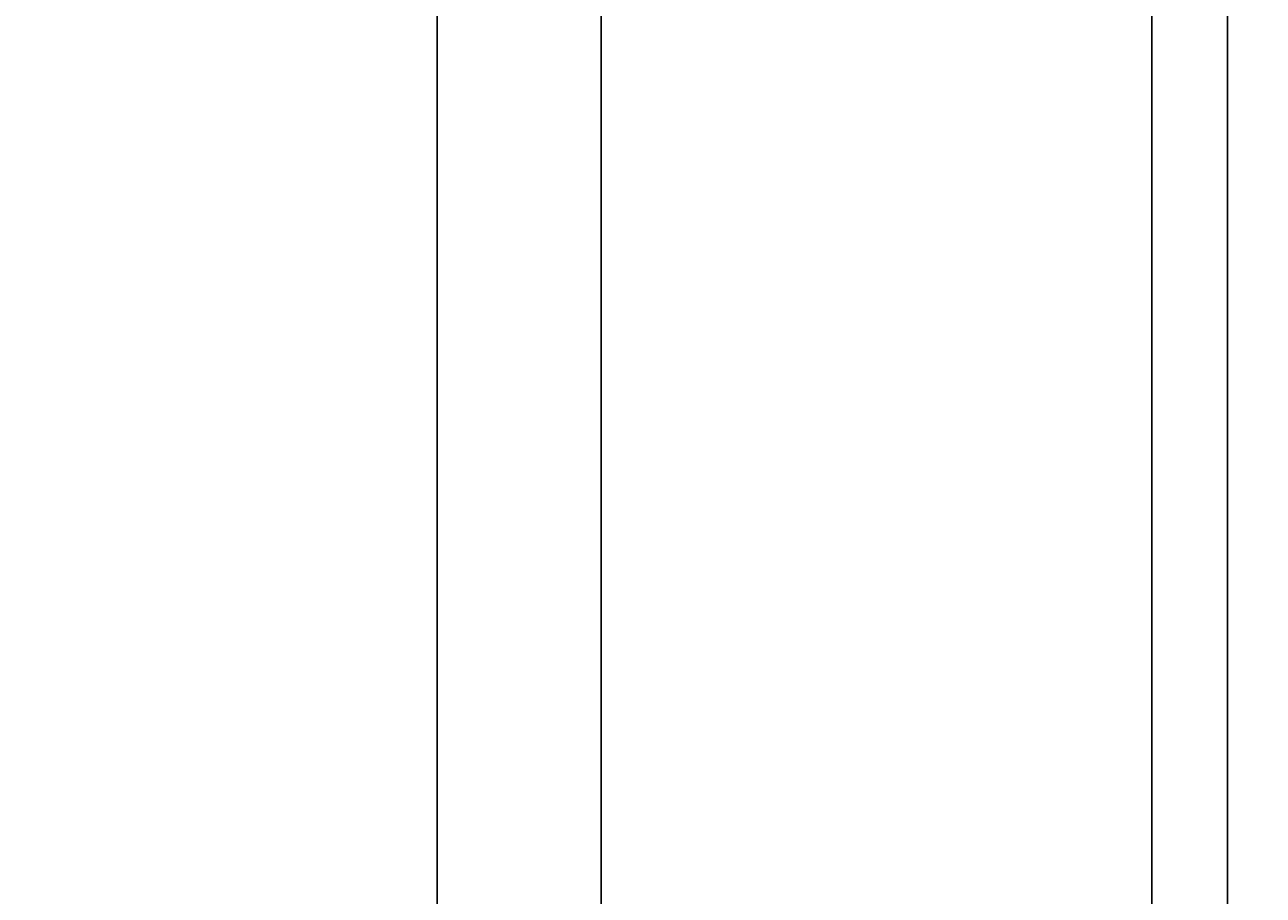
# Model space of a CAD drawing. Units: inches. Extents: x 35362 to 73946, y 43607 to 67532.
# Tile 123 of 134: x 50761 to 51337, y 49329 to 49735. Entities that reach past the tile are written whole.
import ezdxf

# ---------------------------------------------------------------- set-up
doc = ezdxf.new("R2010")
doc.units = ezdxf.units.IN
doc.header["$MEASUREMENT"] = 0
doc.layers.add('A-ANNO-DIMS', color=2, linetype='Continuous', lineweight=18)
doc.styles.get("Standard").update_dxf_attribs({"font": 'arial.ttf'})
doc.dimstyles.get("Standard").update_dxf_attribs({"dimtxt": 0.18, "dimasz": 0.18, "dimexe": 0.18, "dimexo": 0.0625, "dimgap": 0.09, "dimtad": 0, "dimtih": 1, "dimtoh": 1, "dimdec": 4, "dimzin": 0, "dimdsep": 46, "dimtxsty": 'Standard', "dimcen": 0.09, "dimadec": 0, "dimazin": 0, "dimtfac": 1, "dimtdec": 4, "dimtofl": 0, "dimtmove": 0, "dimatfit": 3, "dimfxl": 1, "dimtolj": 1, "dimtzin": 0, "dimarcsym": 0})

# ---------------------------------------------------------------- blocks, each defined once
blk = doc.blocks.new('*D11')
at = {"layer": 'A-ANNO-DIMS', "color": 0, "lineweight": -2, "transparency": 16777216}
for p, q in [((47978.66, 56028.77), (47978.66, 43606.68)), ((53109.76, 56028.77), (53109.76, 43606.68)), ((47978.84, 43606.86), (50543.87, 43606.86)), ((53109.58, 43606.86), (50544.55, 43606.86))]:
    blk.add_line(p, q, dxfattribs=at)
at = {"layer": 'A-ANNO-DIMS', "color": 0, "transparency": 16777216}
for points in [[(47978.84, 43606.89), (47978.84, 43606.83), (47978.66, 43606.86)], [(53109.58, 43606.89), (53109.58, 43606.83), (53109.76, 43606.86)]]:
    blk.add_solid(points, dxfattribs=at)
at = {"layer": 'Defpoints', "color": 0, "transparency": 16777216}
for p in [(47978.66, 56028.84), (53109.76, 56028.84), (53109.76, 43606.86)]:
    blk.add_point(p, dxfattribs=at)
at = {"layer": 'A-ANNO-DIMS', "color": 0, "transparency": 16777216, "insert": (50544.21, 43606.86), "char_height": 0.18, "attachment_point": 5}
blk.add_mtext('\\A1;5131', dxfattribs=at)
blk = doc.blocks.new('*D13')
at = {"layer": 'A-ANNO-DIMS', "color": 0, "lineweight": -2, "transparency": 16777216}
for p, q in [((48373.49, 51694.02), (48373.49, 43606.68)), ((51029.04, 51694.02), (51029.04, 43606.68)), ((48373.67, 43606.86), (49700.8, 43606.86)), ((51028.86, 43606.86), (49701.73, 43606.86))]:
    blk.add_line(p, q, dxfattribs=at)
at = {"layer": 'A-ANNO-DIMS', "color": 0, "transparency": 16777216}
for points in [[(48373.67, 43606.89), (48373.67, 43606.83), (48373.49, 43606.86)], [(51028.86, 43606.89), (51028.86, 43606.83), (51029.04, 43606.86)]]:
    blk.add_solid(points, dxfattribs=at)
at = {"layer": 'Defpoints', "color": 0, "transparency": 16777216}
for p in [(48373.49, 51694.09), (51029.04, 51694.09), (51029.04, 43606.86)]:
    blk.add_point(p, dxfattribs=at)
at = {"layer": 'A-ANNO-DIMS', "color": 0, "transparency": 16777216, "insert": (49701.27, 43606.86), "char_height": 0.18, "attachment_point": 5}
blk.add_mtext('\\A1;2655.6', dxfattribs=at)
blk = doc.blocks.new('*D17')
at = {"layer": 'A-ANNO-DIMS', "color": 0, "lineweight": -2, "transparency": 16777216}
for p, q in [((49923.31, 61293.22), (49923.31, 43606.68)), ((51913.93, 61293.22), (51913.93, 43606.68)), ((49923.49, 43606.86), (50918.16, 43606.86)), ((51913.75, 43606.86), (50919.07, 43606.86))]:
    blk.add_line(p, q, dxfattribs=at)
at = {"layer": 'A-ANNO-DIMS', "color": 0, "transparency": 16777216}
for points in [[(49923.49, 43606.89), (49923.49, 43606.83), (49923.31, 43606.86)], [(51913.75, 43606.89), (51913.75, 43606.83), (51913.93, 43606.86)]]:
    blk.add_solid(points, dxfattribs=at)
at = {"layer": 'Defpoints', "color": 0, "transparency": 16777216}
for p in [(49923.31, 61293.29), (51913.93, 61293.29), (51913.93, 43606.86)]:
    blk.add_point(p, dxfattribs=at)
at = {"layer": 'A-ANNO-DIMS', "color": 0, "transparency": 16777216, "insert": (50918.62, 43606.86), "char_height": 0.18, "attachment_point": 5}
blk.add_mtext('\\A1;1990.6', dxfattribs=at)
blk = doc.blocks.new('*D40')
at = {"layer": 'A-ANNO-DIMS', "color": 0, "lineweight": -2, "transparency": 16777216}
for p, q in [((56873.54, 53351.53), (35361.77, 53351.53)), ((35361.95, 53351.35), (35361.95, 51333.28)), ((35361.95, 49314.85), (35361.95, 51332.92)), ((51806.45, 49314.67), (35361.77, 49314.67))]:
    blk.add_line(p, q, dxfattribs=at)
at = {"layer": 'A-ANNO-DIMS', "color": 0, "transparency": 16777216}
for points in [[(35361.92, 53351.35), (35361.98, 53351.35), (35361.95, 53351.53)], [(35361.92, 49314.85), (35361.98, 49314.85), (35361.95, 49314.67)]]:
    blk.add_solid(points, dxfattribs=at)
at = {"layer": 'Defpoints', "color": 0, "transparency": 16777216}
for p in [(35361.95, 53351.53), (56873.6, 53351.53), (51806.52, 49314.67)]:
    blk.add_point(p, dxfattribs=at)
at = {"layer": 'A-ANNO-DIMS', "color": 0, "transparency": 16777216, "insert": (35361.95, 51333.1), "char_height": 0.18, "attachment_point": 5}
blk.add_mtext('\\A1;4036.9', dxfattribs=at)
blk = doc.blocks.new('*D67')
at = {"layer": 'A-ANNO-DIMS', "color": 0, "lineweight": -2, "transparency": 16777216}
for p, q in [((56873.54, 53351.53), (35361.77, 53351.53)), ((35361.95, 53351.35), (35361.95, 49400.89)), ((35361.95, 45450.07), (35361.95, 49400.53)), ((53793.58, 45449.89), (35361.77, 45449.89))]:
    blk.add_line(p, q, dxfattribs=at)
at = {"layer": 'A-ANNO-DIMS', "color": 0, "transparency": 16777216}
for points in [[(35361.92, 53351.35), (35361.98, 53351.35), (35361.95, 53351.53)], [(35361.92, 45450.07), (35361.98, 45450.07), (35361.95, 45449.89)]]:
    blk.add_solid(points, dxfattribs=at)
at = {"layer": 'Defpoints', "color": 0, "transparency": 16777216}
for p in [(35361.95, 53351.53), (56873.6, 53351.53), (53793.64, 45449.89)]:
    blk.add_point(p, dxfattribs=at)
at = {"layer": 'A-ANNO-DIMS', "color": 0, "transparency": 16777216, "insert": (35361.95, 49400.71), "char_height": 0.18, "attachment_point": 5}
blk.add_mtext('\\A1;7901.6', dxfattribs=at)
blk = doc.blocks.new('*D85')
at = {"layer": 'A-ANNO-DIMS', "color": 0, "lineweight": -2, "transparency": 16777216}
for p, q in [((50952.66, 49098.43), (50952.66, 67531.69)), ((50952.84, 67531.51), (51118.73, 67531.51)), ((51285.41, 67531.51), (51119.52, 67531.51)), ((51285.59, 49320.14), (51285.59, 67531.69))]:
    blk.add_line(p, q, dxfattribs=at)
at = {"layer": 'A-ANNO-DIMS', "color": 0, "transparency": 16777216}
for points in [[(50952.84, 67531.54), (50952.84, 67531.48), (50952.66, 67531.51)], [(51285.41, 67531.54), (51285.41, 67531.48), (51285.59, 67531.51)]]:
    blk.add_solid(points, dxfattribs=at)
at = {"layer": 'Defpoints', "color": 0, "transparency": 16777216}
for p in [(51285.59, 67531.51), (51285.59, 49320.08), (50952.66, 49098.37)]:
    blk.add_point(p, dxfattribs=at)
at = {"layer": 'A-ANNO-DIMS', "color": 0, "transparency": 16777216, "insert": (51119.13, 67531.51), "char_height": 0.18, "attachment_point": 5}
blk.add_mtext('\\A1;332.9', dxfattribs=at)
blk = doc.blocks.new('*D107')
at = {"layer": 'A-ANNO-DIMS', "color": 0, "lineweight": -2, "transparency": 16777216}
for p, q in [((50139.56, 59850.01), (50139.56, 43606.68)), ((51320.81, 59850.01), (51320.81, 43606.68)), ((50139.74, 43606.86), (50729.73, 43606.86)), ((51320.63, 43606.86), (50730.64, 43606.86))]:
    blk.add_line(p, q, dxfattribs=at)
at = {"layer": 'A-ANNO-DIMS', "color": 0, "transparency": 16777216}
for points in [[(50139.74, 43606.89), (50139.74, 43606.83), (50139.56, 43606.86)], [(51320.63, 43606.89), (51320.63, 43606.83), (51320.81, 43606.86)]]:
    blk.add_solid(points, dxfattribs=at)
at = {"layer": 'Defpoints', "color": 0, "transparency": 16777216}
for p in [(50139.56, 59850.08), (51320.81, 59850.08), (51320.81, 43606.86)]:
    blk.add_point(p, dxfattribs=at)
at = {"layer": 'A-ANNO-DIMS', "color": 0, "transparency": 16777216, "insert": (50730.19, 43606.86), "char_height": 0.18, "attachment_point": 5}
blk.add_mtext('\\A1;1181.3', dxfattribs=at)

msp = doc.modelspace()

# ---------------------------------------------------------------- dimensions: what is measured, and where the dimension line sits
at = {"layer": 'A-ANNO-DIMS'}
for base, p1, p2, override, picture, middle in [((51285.595, 67531.512), (50952.662, 49098.368), (51285.595, 49320.079), {"dimdec": 1, "dimlfac": 1, "dimrnd": 0, "dimzin": 0, "dimdsep": 46, "dimlunit": 2}, '*D85', (51119.128, 67531.512)), ((51913.931, 43606.859), (49923.307, 61293.286), (51913.931, 61293.286), {"dimdec": 1, "dimlfac": 1, "dimrnd": 0, "dimzin": 0, "dimdsep": 46, "dimlunit": 2}, '*D17', (50918.619, 43606.859)), ((51320.8133, 43606.859), (50139.5627, 59850.0769), (51320.8133, 59850.0769), {"dimdec": 1, "dimlfac": 1, "dimrnd": 0, "dimzin": 0, "dimdsep": 46, "dimlunit": 2}, '*D107', (50730.188, 43606.859)), ((53109.76, 43606.859), (47978.665, 56028.836), (53109.76, 56028.836), {"dimdec": 0, "dimlfac": 1, "dimrnd": 0, "dimzin": 0, "dimdsep": 46, "dimlunit": 2}, '*D11', (50544.212, 43606.859)), ((51029.043, 43606.859), (48373.492, 51694.087), (51029.043, 51694.087), {"dimdec": 1, "dimlfac": 1, "dimrnd": 0, "dimzin": 0, "dimdsep": 46, "dimlunit": 2}, '*D13', (49701.267, 43606.859))]:
    dim = msp.add_linear_dim(base=base, p1=p1, p2=p2, dimstyle='Standard', override=override, dxfattribs=at)
    dim.commit()
    dim.dimension.update_dxf_attribs({"geometry": picture, "text_midpoint": middle})
for p1, picture, middle in [((51806.517, 49314.669), '*D40', (35361.949, 51333.099)), ((53793.638, 45449.894), '*D67', (35361.949, 49400.712))]:
    dim = msp.add_linear_dim(base=(35361.949, 53351.529), p1=p1, p2=(56873.602, 53351.529), angle=90, dimstyle='Standard', override={"dimdec": 1, "dimlfac": 1, "dimrnd": 0, "dimzin": 0, "dimdsep": 46, "dimlunit": 2}, dxfattribs=at)
    dim.commit()
    dim.dimension.update_dxf_attribs({"geometry": picture, "text_midpoint": middle})

doc.saveas('drawing.dxf')
